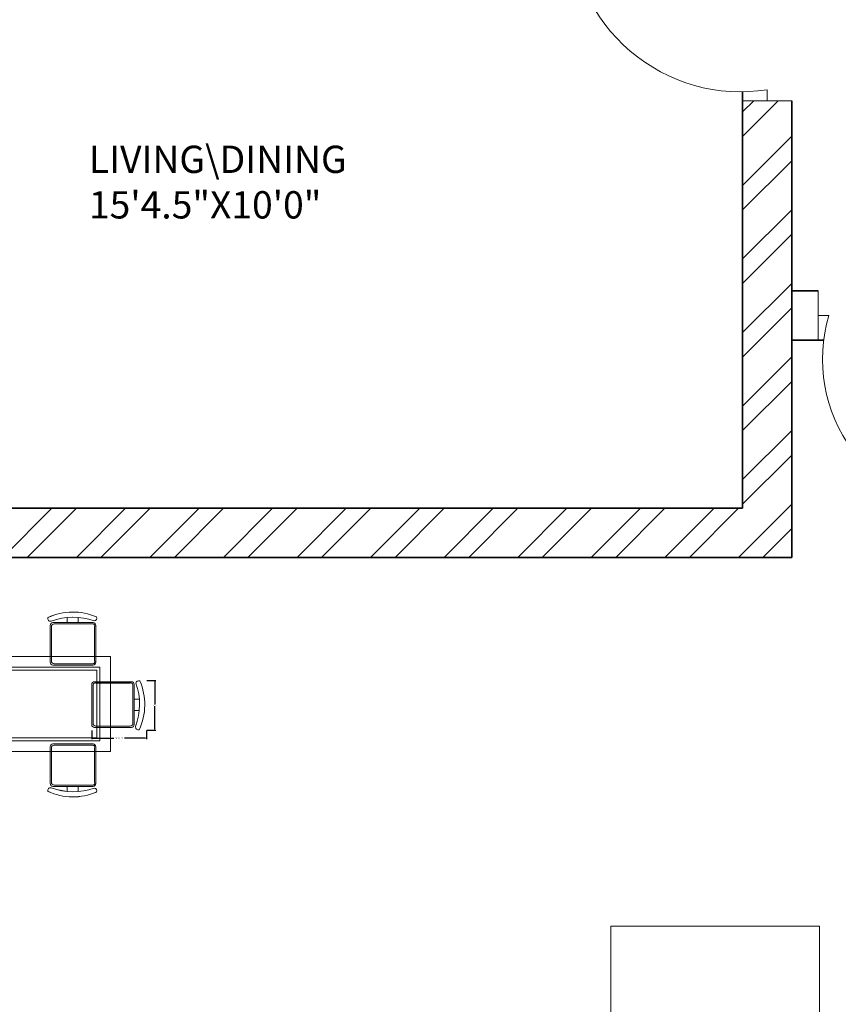
# Model space of a CAD drawing. Units: inches. Extents: x 2120 to 4013, y 1390 to 3019.
# Tile 14 of 59: x 2448 to 2598, y 1784 to 1964. Entities that reach past the tile are written whole.
import ezdxf

# ---------------------------------------------------------------- set-up
doc = ezdxf.new("R2010")
doc.units = ezdxf.units.IN
for name, color, linetype, lineweight in [('A-ANNO-DIMS', 2, 'Continuous', 18), ('A-AREA-IDEN', 7, 'Continuous', 18), ('A-DOOR', 3, 'Continuous', 18), ('A-FURN', 8, 'Continuous', 13), ('A-WALL', 7, 'Continuous', 35), ('A-WALL-PATT', 252, 'Continuous', 13)]:
    doc.layers.add(name, color=color, linetype=linetype, lineweight=lineweight)
doc.styles.get("Standard").update_dxf_attribs({"font": 'arial.ttf'})
doc.dimstyles.get("Standard").update_dxf_attribs({"dimtxt": 0.18, "dimasz": 0.18, "dimexe": 0.18, "dimexo": 0.0625, "dimgap": 0.09, "dimtad": 0, "dimtih": 1, "dimtoh": 1, "dimdec": 4, "dimzin": 0, "dimdsep": 46, "dimtxsty": 'Standard', "dimcen": 0.09, "dimadec": 0, "dimazin": 0, "dimtfac": 1, "dimtdec": 4, "dimtofl": 0, "dimtmove": 0, "dimatfit": 3, "dimfxl": 1, "dimtolj": 1, "dimtzin": 0, "dimarcsym": 0})

# ---------------------------------------------------------------- blocks, each defined once
blk = doc.blocks.new('DOOR-SWING-36IN-98p95DEG')
for p, q in [((31.5, 34.77), (40.5, 34.77)), ((40.5, 34.77), (36, 34.77)), ((36, 34.77), (36, 32.77)), ((36, 32.77), (0, 32.77)), ((36, 0), (36, 2)), ((31.5, 0), (40.5, 0)), ((40.5, 0), (36, 0))]:
    blk.add_line(p, q)
blk.add_arc((31.15, 32.77), 31.15, 180, 278.9496)
blk = doc.blocks.new('DOOR-SWING-36IN-106p79DEG')
for p, q in [((0, 40.5), (0, 31.5)), ((30.74, 31.5), (30.74, 40.5)), ((30.74, 40.5), (30.74, 36)), ((0, 31.5), (0, 36)), ((0, 36), (2, 36)), ((30.74, 36), (28.74, 36)), ((28.74, 36), (28.74, 0))]:
    blk.add_line(p, q)
blk.add_arc((28.74, 27.93), 27.93, 163.2075, 270)
blk = doc.blocks.new('TABLE-DINING')
for points in [[(0, 17.41), (29.01, 17.41), (29.01, 0), (0, 0)], [(1.93, 15.47), (27.08, 15.47), (27.08, 1.93), (1.93, 1.93)], [(2.51, 14.89), (26.5, 14.89), (26.5, 2.51), (2.51, 2.51)]]:
    blk.add_lwpolyline(points, close=True)
blk = doc.blocks.new('TABLE-COFFEE')
blk.add_lwpolyline([(0, 38.19), (21.88, 38.19), (21.88, 0), (0, 0)], close=True)
blk = doc.blocks.new('CHAIR-DINING-01')
for points in [[(1.68, 0.62, -0.578392), (1.02, 0.02, -0.214524), (0.9, 8.94, -0.552014), (1.62, 8.52, 0.175809), (1.68, 0.62)], [(1.93, 8.29, -0.414214), (2.45, 8.81), (9.19, 8.81, -0.414214), (9.7, 8.29), (9.7, 0.96, -0.414214), (9.19, 0.45), (2.45, 0.45, -0.414214), (1.93, 0.96), (1.93, 8.29)], [(1.93, 3.54), (1.01, 3.54, 0.064759)]]:
    blk.add_lwpolyline(points, format="xyb")
blk.add_lwpolyline([(2.16, 8.29), (2.16, 1.19, 0.414214), (2.68, 0.68), (8.96, 0.68, 0.414214), (9.47, 1.19), (9.47, 8.29, 0.512069), (8.96, 8.58), (2.68, 8.58, 0.512069)], format="xyb", close=True)
blk.add_lwpolyline([(0.99, 5.59), (1.93, 5.59)])
blk = doc.blocks.new('CHAIR-DINING-02')
for points in [[(7.77, 8.29, 0.414214), (7.26, 8.81), (0.51, 8.81, 0.414214), (0, 8.29), (0, 0.96, 0.414214), (0.51, 0.45), (7.26, 0.45, 0.414214), (7.77, 0.96), (7.77, 8.29)], [(8.09, 8.52, -0.175809), (8.03, 0.62, 0.578392), (8.69, 0.02, 0.214524), (8.81, 8.94, 0.552014), (8.09, 8.52, -0.065079)], [(7.77, 3.54), (8.7, 3.54, -0.064759)]]:
    blk.add_lwpolyline(points, format="xyb")
blk.add_lwpolyline([(7.54, 8.29), (7.54, 1.19, -0.414214), (7.03, 0.68), (0.74, 0.68, -0.414214), (0.23, 1.19), (0.23, 8.29, -0.512069), (0.74, 8.58), (7.03, 8.58, -0.512069)], format="xyb", close=True)
blk.add_lwpolyline([(8.72, 5.59), (7.77, 5.59)])
blk = doc.blocks.new('CHAIR-DINING-03')
for points in [[(8.29, 1.93, 0.414214), (8.81, 2.45), (8.81, 9.19, 0.414214), (8.29, 9.7), (0.96, 9.7, 0.414214), (0.45, 9.19), (0.45, 2.45, 0.414214), (0.96, 1.93), (8.29, 1.93)], [(3.54, 1.93), (3.54, 1.01, -0.064759)], [(8.52, 1.62, -0.175809), (0.62, 1.68, 0.578392), (0.02, 1.02, 0.214524), (8.94, 0.9, 0.552014), (8.52, 1.62, -0.065079)]]:
    blk.add_lwpolyline(points, format="xyb")
blk.add_lwpolyline([(8.29, 2.16), (1.19, 2.16, -0.414214), (0.68, 2.68), (0.68, 8.96, -0.414214), (1.19, 9.47), (8.29, 9.47, -0.512069), (8.58, 8.96), (8.58, 2.68, -0.512069)], format="xyb", close=True)
blk.add_lwpolyline([(5.59, 0.99), (5.59, 1.93)])
blk = doc.blocks.new('*D83')
at = {"layer": 'A-ANNO-DIMS', "color": 0, "lineweight": -2, "transparency": 16777216}
for p, q in [((2461.05, 1833.87), (2461.05, 1832.25)), ((2471.1, 1833.87), (2471.1, 1832.25)), ((2461.23, 1832.43), (2465.12, 1832.43)), ((2470.92, 1832.43), (2467.03, 1832.43))]:
    blk.add_line(p, q, dxfattribs=at)
at = {"layer": 'A-ANNO-DIMS', "color": 0, "transparency": 16777216}
for points in [[(2461.23, 1832.46), (2461.23, 1832.4), (2461.05, 1832.43)], [(2470.92, 1832.46), (2470.92, 1832.4), (2471.1, 1832.43)]]:
    blk.add_solid(points, dxfattribs=at)
at = {"layer": 'Defpoints', "color": 0, "transparency": 16777216}
for p in [(2461.05, 1833.93), (2471.1, 1833.93), (2471.1, 1832.43)]:
    blk.add_point(p, dxfattribs=at)
at = {"layer": 'A-ANNO-DIMS', "color": 0, "transparency": 16777216, "insert": (2466.08, 1832.43), "char_height": 0.18, "attachment_point": 5}
blk.add_mtext('\\A1;CHAIR 10 TYP.', dxfattribs=at)
blk = doc.blocks.new('*D84')
at = {"layer": 'A-ANNO-DIMS', "color": 0, "lineweight": -2, "transparency": 16777216}
for p, q in [((2471.16, 1842.99), (2472.78, 1842.99)), ((2472.6, 1842.81), (2472.6, 1838.64)), ((2472.6, 1834.11), (2472.6, 1838.28)), ((2471.16, 1833.93), (2472.78, 1833.93))]:
    blk.add_line(p, q, dxfattribs=at)
at = {"layer": 'A-ANNO-DIMS', "color": 0, "transparency": 16777216}
for points in [[(2472.57, 1842.81), (2472.63, 1842.81), (2472.6, 1842.99)], [(2472.57, 1834.11), (2472.63, 1834.11), (2472.6, 1833.93)]]:
    blk.add_solid(points, dxfattribs=at)
at = {"layer": 'Defpoints', "color": 0, "transparency": 16777216}
for p in [(2471.1, 1842.99), (2472.6, 1842.99), (2471.1, 1833.93)]:
    blk.add_point(p, dxfattribs=at)
at = {"layer": 'A-ANNO-DIMS', "color": 0, "transparency": 16777216, "insert": (2472.6, 1838.46), "char_height": 0.18, "attachment_point": 5}
blk.add_mtext('\\A1;9 TYP.', dxfattribs=at)

msp = doc.modelspace()

# ---------------------------------------------------------------- hatches: boundary and pattern name
at = {"layer": 'A-WALL-PATT'}
h = msp.add_hatch(dxfattribs=at)
h.set_pattern_fill('ANSI32', color=256)
h.paths.add_polyline_path([(2271.7331, 2343.531), (2283.3788, 2343.531), (2283.3788, 2348.031), (2283.3788, 2352.5306), (2262.7331, 2352.5306), (2262.7331, 2182.638), (2267.2331, 2182.638), (2271.7331, 2182.638), (2271.7331, 2219.031), (2391.7331, 2219.031), (2391.7331, 2214.189), (2393.9831, 2214.189), (2396.2331, 2214.189), (2396.2331, 2219.031), (2420.2331, 2219.031), (2420.2331, 2225.7535), (2417.2197, 2225.7535), (2415.7331, 2225.7535), (2415.7331, 2223.5306), (2271.7331, 2223.5306)])
h.paths.add_polyline_path([(2380.0942, 2352.5306), (2343.3788, 2352.5306), (2343.3788, 2343.531), (2363.2331, 2343.531), (2363.2331, 2288.8489), (2365.4831, 2288.8489), (2367.7331, 2288.8489), (2367.7331, 2343.531), (2380.0942, 2343.531)], flags=17)
h.paths.add_polyline_path([(2432.4339, 2352.5306), (2404.0943, 2352.5306), (2404.0943, 2343.531), (2415.7331, 2343.531), (2415.7331, 2264.0306), (2367.7331, 2264.0306), (2367.7331, 2266.4872), (2363.2331, 2266.4872), (2363.2331, 2259.531), (2367.7331, 2259.531), (2415.7331, 2259.531), (2415.7331, 2255.0658), (2420.2331, 2255.0658), (2420.2331, 2259.531), (2424.5717, 2259.531), (2424.5717, 2261.781), (2424.5717, 2264.0306), (2420.2331, 2264.0306), (2420.2331, 2343.531), (2432.4339, 2343.531)])
h.paths.add_polyline_path([(2508.9115, 2352.5306), (2456.4339, 2352.5306), (2456.4339, 2343.531), (2468.2331, 2343.531), (2468.2331, 2264.0306), (2448.0487, 2264.0306), (2448.0487, 2259.531), (2468.2331, 2259.531), (2468.2331, 2255.5496), (2472.7331, 2255.5496), (2472.7331, 2343.531), (2508.9115, 2343.531)])
h.paths.add_polyline_path([(2637.7331, 2352.5306), (2544.9116, 2352.5306), (2544.9116, 2343.531), (2589.7331, 2343.531), (2633.2331, 2343.531), (2637.7331, 2343.531)])
h.paths.add_polyline_path([(2594.2331, 2343.5306), (2589.7331, 2343.5306), (2589.7331, 2259.5306), (2589.7331, 2252.4915), (2591.9831, 2252.4915), (2594.2331, 2252.4915)])
h.paths.add_polyline_path([(2637.7331, 2223.5306), (2594.2331, 2223.5306), (2594.2331, 2230.1988), (2591.9831, 2230.1988), (2589.7331, 2230.1988), (2589.7331, 2223.5306), (2472.7331, 2223.5306), (2468.2331, 2223.5306), (2468.2331, 2219.031), (2628.7331, 2219.031), (2628.7331, 2138.031), (2637.7331, 2138.031)])
h.paths.add_polyline_path([(3822.6535, 2458.4402), (3874.9468, 2458.4402), (3874.9468, 2476.9866), (3822.6535, 2476.9866)], flags=9)
h.paths.add_polyline_path([(3834.6921, 2781.8174), (3935.9206, 2781.8174), (3935.9206, 2800.3638), (3834.6921, 2800.3638)], flags=9)
h.paths.add_polyline_path([(3832.2843, 2837.9683), (3884.5776, 2837.9683), (3884.5776, 2856.5146), (3832.2843, 2856.5146)], flags=9)
h.paths.add_polyline_path([(3830.9388, 2861.4782), (3956.8958, 2861.4782), (3956.8958, 2880.0245), (3830.9388, 2880.0245)], flags=9)
h.paths.add_polyline_path([(3870.6966, 2352.5752), (3887.9272, 2352.5752), (3887.9272, 2377.3037), (3870.6966, 2377.3037)], flags=9)
h.paths.add_polyline_path([(3289.2701, 2413.161), (3435.2223, 2413.161), (3435.2223, 2450.2538), (3289.2701, 2450.2538)], flags=9)
h.paths.add_polyline_path([(2487.6944, 2414.3601), (2637.8335, 2414.3601), (2637.8335, 2451.4528), (2487.6944, 2451.4528)], flags=9)
h.paths.add_polyline_path([(2567.3724, 1457.9199), (2815.296, 1457.9199), (2815.296, 1495.0127), (2567.3724, 1495.0127)], flags=9)
h.paths.add_polyline_path([(2655.3825, 2093.2363), (2685.9555, 2093.2363), (2685.9555, 2111.8937), (2655.3825, 2111.8937)], flags=9)
h.paths.add_polyline_path([(2543.9218, 1550.6671), (2587.8406, 1550.6671), (2587.8406, 1569.3244), (2543.9218, 1569.3244)], flags=9)
h.paths.add_polyline_path([(2905.1384, 1543.8113), (2949.0572, 1543.8113), (2949.0572, 1562.4686), (2905.1384, 1562.4686)], flags=9)
h.paths.add_polyline_path([(2736.4118, 1702.4736), (2784.2153, 1702.4736), (2784.2153, 1721.1309), (2736.4118, 1721.1309)], flags=9)
h.paths.add_polyline_path([(2912.8666, 1710.4168), (2951.707, 1710.4168), (2951.707, 1729.0741), (2912.8666, 1729.0741)], flags=9)
h.paths.add_polyline_path([(2923.5785, 1763.5038), (2959.7279, 1763.5038), (2959.7279, 1782.1611), (2923.5785, 1782.1611)], flags=9)
h.paths.add_polyline_path([(2925.2114, 1809.6137), (2967.1861, 1809.6137), (2967.1861, 1828.271), (2925.2114, 1828.271)], flags=9)
h.paths.add_polyline_path([(2996.2711, 1878.9003), (2996.2711, 1913.109), (2977.6138, 1913.109), (2977.6138, 1878.9003)], flags=9)
h.paths.add_polyline_path([(2883.0859, 1895.7192), (2927.1855, 1895.7192), (2927.1855, 1914.3766), (2883.0859, 1914.3766)], flags=9)
h.paths.add_polyline_path([(2787.3924, 1810.8013), (2841.0213, 1810.8013), (2841.0213, 1829.4587), (2787.3924, 1829.4587)], flags=9)
h.paths.add_polyline_path([(2775.6399, 2101.7395), (2829.2689, 2101.7395), (2829.2689, 2120.3968), (2775.6399, 2120.3968)], flags=9)
h.paths.add_polyline_path([(2913.0263, 2075.817), (2951.8667, 2075.817), (2951.8667, 2094.4744), (2913.0263, 2094.4744)], flags=9)
h.paths.add_polyline_path([(2929.966, 2133.3669), (2966.1154, 2133.3669), (2966.1154, 2152.0243), (2929.966, 2152.0243)], flags=9)
h.paths.add_polyline_path([(2932.7502, 2182.6088), (2968.8996, 2182.6088), (2968.8996, 2201.2662), (2932.7502, 2201.2662)], flags=9)
h.paths.add_polyline_path([(2996.0681, 2266.3173), (2996.0681, 2300.5261), (2977.4108, 2300.5261), (2977.4108, 2266.3173)], flags=9)
h.paths.add_polyline_path([(2885.1039, 2279.2186), (2929.2035, 2279.2186), (2929.2035, 2297.8759), (2885.1039, 2297.8759)], flags=9)
h.paths.add_polyline_path([(2735.7042, 2218.3197), (2783.5078, 2218.3197), (2783.5078, 2236.9771), (2735.7042, 2236.9771)], flags=9)
h.paths.add_polyline_path([(2635.6049, 2044.0085), (2648.9678, 2044.0085), (2648.9678, 2054.312), (2635.6049, 2054.312)], flags=9)
h.paths.add_polyline_path([(2714.0148, 1923.0473), (2727.3777, 1923.0473), (2727.3777, 1933.3508), (2714.0148, 1933.3508)], flags=9)
h.paths.add_polyline_path([(2709.0345, 1988.1628), (2722.3974, 1988.1628), (2722.3974, 1998.4663), (2709.0345, 1998.4663)], flags=9)
h.paths.add_polyline_path([(2592.8935, 1962.1763), (2606.2564, 1962.1763), (2606.2564, 1972.4799), (2592.8935, 1972.4799)], flags=9)
h.paths.add_polyline_path([(2618.3996, 1985.9724), (2644.1942, 1985.9724), (2644.1942, 1996.2759), (2618.3996, 1996.2759)], flags=9)
h.paths.add_polyline_path([(2601.279, 1920.5869), (2614.6419, 1920.5869), (2614.6419, 1930.8904), (2601.279, 1930.8904)], flags=9)
h.paths.add_polyline_path([(2692.3278, 1932.7645), (2704.5311, 1932.7645), (2704.5311, 1943.0681), (2692.3278, 1943.0681)], flags=9)
h.paths.add_polyline_path([(2311.122, 1672.7318), (2355.0408, 1672.7318), (2355.0408, 1691.3892), (2311.122, 1691.3892)], flags=9)
h.paths.add_polyline_path([(2456.2551, 1632.3198), (2492.4796, 1632.3198), (2492.4796, 1650.9772), (2456.2551, 1650.9772)], flags=9)
h.paths.add_polyline_path([(2401.0766, 1631.4793), (2437.301, 1631.4793), (2437.301, 1650.1367), (2401.0766, 1650.1367)], flags=9)
h.paths.add_polyline_path([(2546.7054, 1700.9235), (2594.509, 1700.9235), (2594.509, 1719.5809), (2546.7054, 1719.5809)], flags=9)
h.paths.add_polyline_path([(2445.4866, 1766.9937), (2497.5261, 1766.9937), (2497.5261, 1785.651), (2445.4866, 1785.651)], flags=9)
h.paths.add_polyline_path([(2287.9992, 1739.7675), (2326.8396, 1739.7675), (2326.8396, 1758.4248), (2287.9992, 1758.4248)], flags=9)
h.paths.add_polyline_path([(2458.5279, 1924.7607), (2510.5675, 1924.7607), (2510.5675, 1943.4181), (2458.5279, 1943.4181)], flags=9)
h.paths.add_polyline_path([(2309.2811, 1902.7642), (2345.4305, 1902.7642), (2345.4305, 1921.4215), (2309.2811, 1921.4215)], flags=9)
h.paths.add_polyline_path([(2490.7554, 2018.9392), (2530.7896, 2018.9392), (2530.7896, 2037.5965), (2490.7554, 2037.5965)], flags=9)
h.paths.add_polyline_path([(2402.143, 2024.7393), (2438.5414, 2024.7393), (2438.5414, 2043.3966), (2402.143, 2043.3966)], flags=9)
h.paths.add_polyline_path([(2287.856, 1931.7926), (2326.6964, 1931.7926), (2326.6964, 1950.4499), (2287.856, 1950.4499)], flags=9)
h.paths.add_polyline_path([(2281.7979, 2193.5771), (2320.6383, 2193.5771), (2320.6383, 2212.2344), (2281.7979, 2212.2344)], flags=25)
h.paths.add_polyline_path([(2484.0754, 2093.892), (2536.115, 2093.892), (2536.115, 2112.5494), (2484.0754, 2112.5494)], flags=9)
h.paths.add_polyline_path([(2624.7948, 2281.8639), (2624.7948, 2311.4137), (2606.1375, 2311.4137), (2606.1375, 2281.8639)], flags=9)
h.paths.add_polyline_path([(2507.5036, 2290.3639), (2541.934, 2290.3639), (2541.934, 2309.0212), (2507.5036, 2309.0212)], flags=9)
h.paths.add_polyline_path([(2423.1076, 2285.2202), (2459.332, 2285.2202), (2459.332, 2303.8776), (2423.1076, 2303.8776)], flags=9)
h.paths.add_polyline_path([(2374.5467, 2289.6272), (2410.7711, 2289.6272), (2410.7711, 2308.2846), (2374.5467, 2308.2846)], flags=25)
h.paths.add_polyline_path([(2277.4907, 2227.5651), (2316.3311, 2227.5651), (2316.3311, 2246.2224), (2277.4907, 2246.2224)], flags=25)
h.paths.add_polyline_path([(2655.3825, 2093.2367), (2685.9555, 2093.2367), (2685.9555, 2111.894), (2655.3825, 2111.894)], flags=9)
h.paths.add_polyline_path([(2543.9217, 1550.6674), (2587.8406, 1550.6674), (2587.8406, 1569.3247), (2543.9217, 1569.3247)], flags=9)
h.paths.add_polyline_path([(2905.1384, 1543.8116), (2949.0572, 1543.8116), (2949.0572, 1562.4689), (2905.1384, 1562.4689)], flags=9)
h.paths.add_polyline_path([(2736.4118, 1702.4739), (2784.2153, 1702.4739), (2784.2153, 1721.1312), (2736.4118, 1721.1312)], flags=9)
h.paths.add_polyline_path([(2912.8666, 1710.4171), (2951.707, 1710.4171), (2951.707, 1729.0744), (2912.8666, 1729.0744)], flags=9)
h.paths.add_polyline_path([(2923.5785, 1763.5041), (2959.7279, 1763.5041), (2959.7279, 1782.1614), (2923.5785, 1782.1614)], flags=9)
h.paths.add_polyline_path([(2925.2114, 1809.614), (2967.1861, 1809.614), (2967.1861, 1828.2713), (2925.2114, 1828.2713)], flags=9)
h.paths.add_polyline_path([(2996.2711, 1878.9006), (2996.2711, 1913.1094), (2977.6137, 1913.1094), (2977.6137, 1878.9006)], flags=9)
h.paths.add_polyline_path([(2883.0859, 1895.7195), (2927.1855, 1895.7195), (2927.1855, 1914.3769), (2883.0859, 1914.3769)], flags=9)
h.paths.add_polyline_path([(2787.3924, 1810.8016), (2841.0213, 1810.8016), (2841.0213, 1829.459), (2787.3924, 1829.459)], flags=9)
h.paths.add_polyline_path([(2775.6399, 2101.7398), (2829.2688, 2101.7398), (2829.2688, 2120.3971), (2775.6399, 2120.3971)], flags=9)
h.paths.add_polyline_path([(2913.0263, 2075.8173), (2951.8667, 2075.8173), (2951.8667, 2094.4747), (2913.0263, 2094.4747)], flags=9)
h.paths.add_polyline_path([(2929.966, 2133.3672), (2966.1154, 2133.3672), (2966.1154, 2152.0246), (2929.966, 2152.0246)], flags=9)
h.paths.add_polyline_path([(2932.7502, 2182.6091), (2968.8996, 2182.6091), (2968.8996, 2201.2665), (2932.7502, 2201.2665)], flags=9)
h.paths.add_polyline_path([(2996.0681, 2266.3176), (2996.0681, 2300.5264), (2977.4108, 2300.5264), (2977.4108, 2266.3176)], flags=9)
h.paths.add_polyline_path([(2885.1039, 2279.2189), (2929.2035, 2279.2189), (2929.2035, 2297.8762), (2885.1039, 2297.8762)], flags=9)
h.paths.add_polyline_path([(2735.7042, 2218.32), (2783.5078, 2218.32), (2783.5078, 2236.9774), (2735.7042, 2236.9774)], flags=9)
h.paths.add_polyline_path([(2635.6048, 2044.0088), (2648.9677, 2044.0088), (2648.9677, 2054.3123), (2635.6048, 2054.3123)], flags=9)
h.paths.add_polyline_path([(2714.0148, 1923.0476), (2727.3777, 1923.0476), (2727.3777, 1933.3511), (2714.0148, 1933.3511)], flags=9)
h.paths.add_polyline_path([(2709.0345, 1988.1631), (2722.3974, 1988.1631), (2722.3974, 1998.4666), (2709.0345, 1998.4666)], flags=9)
h.paths.add_polyline_path([(2592.8935, 1962.1766), (2606.2564, 1962.1766), (2606.2564, 1972.4802), (2592.8935, 1972.4802)], flags=9)
h.paths.add_polyline_path([(2618.3995, 1985.9727), (2644.1942, 1985.9727), (2644.1942, 1996.2762), (2618.3995, 1996.2762)], flags=9)
h.paths.add_polyline_path([(2601.279, 1920.5872), (2614.6419, 1920.5872), (2614.6419, 1930.8908), (2601.279, 1930.8908)], flags=9)
h.paths.add_polyline_path([(2692.3278, 1932.7648), (2704.5311, 1932.7648), (2704.5311, 1943.0684), (2692.3278, 1943.0684)], flags=9)
h.paths.add_polyline_path([(2311.122, 1672.7321), (2355.0408, 1672.7321), (2355.0408, 1691.3895), (2311.122, 1691.3895)], flags=9)
h.paths.add_polyline_path([(2456.2551, 1632.3201), (2492.4795, 1632.3201), (2492.4795, 1650.9775), (2456.2551, 1650.9775)], flags=9)
h.paths.add_polyline_path([(2401.0766, 1631.4796), (2437.301, 1631.4796), (2437.301, 1650.137), (2401.0766, 1650.137)], flags=9)
h.paths.add_polyline_path([(2546.7054, 1700.9238), (2594.509, 1700.9238), (2594.509, 1719.5812), (2546.7054, 1719.5812)], flags=9)
h.paths.add_polyline_path([(2445.4866, 1766.994), (2497.5261, 1766.994), (2497.5261, 1785.6513), (2445.4866, 1785.6513)], flags=9)
h.paths.add_polyline_path([(2287.9992, 1739.7678), (2326.8396, 1739.7678), (2326.8396, 1758.4251), (2287.9992, 1758.4251)], flags=9)
h.paths.add_polyline_path([(2458.5279, 1924.7611), (2510.5675, 1924.7611), (2510.5675, 1943.4184), (2458.5279, 1943.4184)], flags=9)
h.paths.add_polyline_path([(2309.2811, 1902.7645), (2345.4305, 1902.7645), (2345.4305, 1921.4218), (2309.2811, 1921.4218)], flags=9)
h.paths.add_polyline_path([(2490.7554, 2018.9395), (2530.7895, 2018.9395), (2530.7895, 2037.5968), (2490.7554, 2037.5968)], flags=9)
h.paths.add_polyline_path([(2402.143, 2024.7396), (2438.5413, 2024.7396), (2438.5413, 2043.3969), (2402.143, 2043.3969)], flags=9)
h.paths.add_polyline_path([(2287.856, 1931.7929), (2326.6964, 1931.7929), (2326.6964, 1950.4502), (2287.856, 1950.4502)], flags=9)
h.paths.add_polyline_path([(2281.7979, 2193.5774), (2320.6383, 2193.5774), (2320.6383, 2212.2347), (2281.7979, 2212.2347)], flags=25)
h.paths.add_polyline_path([(2484.0754, 2093.8924), (2536.115, 2093.8924), (2536.115, 2112.5497), (2484.0754, 2112.5497)], flags=9)
h.paths.add_polyline_path([(2624.7948, 2281.8642), (2624.7948, 2311.414), (2606.1374, 2311.414), (2606.1374, 2281.8642)], flags=9)
h.paths.add_polyline_path([(2507.5035, 2290.3642), (2541.934, 2290.3642), (2541.934, 2309.0215), (2507.5035, 2309.0215)], flags=9)
h.paths.add_polyline_path([(2423.1075, 2285.2205), (2459.332, 2285.2205), (2459.332, 2303.8779), (2423.1075, 2303.8779)], flags=9)
h.paths.add_polyline_path([(2374.5467, 2289.6275), (2410.7711, 2289.6275), (2410.7711, 2308.2849), (2374.5467, 2308.2849)], flags=25)
h.paths.add_polyline_path([(2277.4907, 2227.5654), (2316.3311, 2227.5654), (2316.3311, 2246.2227), (2277.4907, 2246.2227)], flags=25)
h = msp.add_hatch(dxfattribs=at)
h.set_pattern_fill('ANSI32', color=256)
h.paths.add_polyline_path([(2271.7331, 1980.389), (2262.7331, 1980.389), (2262.7331, 1912.8434), (2267.2331, 1912.8434), (2271.7331, 1912.8434), (2271.7331, 1922.531), (2351.2331, 1922.531), (2351.2331, 1901.4728), (2355.7331, 1901.4728), (2355.7331, 1922.531), (2357.9815, 1922.531), (2357.9815, 1926.5306), (2271.7331, 1926.5306)])
h.paths.add_polyline_path([(2589.2331, 1949.1622), (2584.7331, 1949.1622), (2580.2331, 1949.1622), (2580.2331, 1874.5306), (2355.7331, 1874.5306), (2355.7331, 1880.1922), (2351.2331, 1880.1922), (2351.2331, 1874.5306), (2271.7331, 1874.5306), (2271.7331, 1888.8431), (2262.7331, 1888.8431), (2262.7331, 1842.2909), (2267.2331, 1842.2909), (2271.7331, 1842.2909), (2271.7331, 1865.531), (2415.7331, 1865.531), (2415.7331, 1779.7286), (2420.2331, 1779.7286), (2420.2331, 1865.531), (2589.2331, 1865.531)])
h.paths.add_polyline_path([(2271.7331, 1782.2906), (2262.7331, 1782.2906), (2262.7331, 1711.4639), (2267.2331, 1711.4639), (2271.7331, 1711.4639), (2271.7331, 1738.031), (2420.2331, 1738.031), (2420.2331, 1742.531), (2420.2331, 1747.3376), (2417.9831, 1747.3376), (2415.7331, 1747.3376), (2415.7331, 1742.5306), (2271.7331, 1742.5306)])
h.paths.add_polyline_path([(2271.7331, 1627.031), (2362.3957, 1627.031), (2362.3957, 1629.281), (2362.3957, 1631.5306), (2271.7331, 1631.5306), (2271.7331, 1675.4636), (2262.7331, 1675.4636), (2262.7331, 1581.531), (2405.3032, 1581.531), (2405.3032, 1586.031), (2405.3032, 1590.5306), (2396.2331, 1590.5306), (2396.2331, 1691.4513), (2418.7206, 1691.4513), (2418.7206, 1695.951), (2396.2331, 1695.951), (2391.7331, 1695.951), (2391.7331, 1631.5306), (2386.7425, 1631.5306), (2386.7425, 1629.2806), (2386.7425, 1627.031), (2391.7331, 1627.031), (2391.7331, 1586.1709), (2271.7331, 1586.1709)])
h.paths.add_polyline_path([(2459.6703, 1590.5306), (2429.3032, 1590.5306), (2429.3032, 1581.531), (2459.6703, 1581.531), (2459.6703, 1586.031)])
h.paths.add_polyline_path([(2501.2331, 1590.531), (2501.2331, 1665.0195), (2498.9831, 1665.0195), (2496.7331, 1665.0195), (2496.7331, 1590.5306), (2483.8201, 1590.5306), (2483.8201, 1590.1579), (2483.6704, 1590.1579), (2483.6704, 1581.531), (2505.0196, 1581.531), (2505.0196, 1583.781), (2505.0196, 1586.0306), (2501.2331, 1586.0306)])
h.paths.add_polyline_path([(2544.1361, 1583.781), (2544.1361, 1586.0306), (2527.1368, 1586.0306), (2527.1368, 1583.7806), (2527.1368, 1581.531), (2544.1361, 1581.531)])
h.paths.add_polyline_path([(3822.6535, 2458.4402), (3874.9468, 2458.4402), (3874.9468, 2476.9866), (3822.6535, 2476.9866)], flags=9)
h.paths.add_polyline_path([(3834.6921, 2781.8174), (3935.9206, 2781.8174), (3935.9206, 2800.3638), (3834.6921, 2800.3638)], flags=9)
h.paths.add_polyline_path([(3832.2843, 2837.9683), (3884.5776, 2837.9683), (3884.5776, 2856.5146), (3832.2843, 2856.5146)], flags=9)
h.paths.add_polyline_path([(3830.9388, 2861.4782), (3956.8958, 2861.4782), (3956.8958, 2880.0245), (3830.9388, 2880.0245)], flags=9)
h.paths.add_polyline_path([(3870.6966, 2352.5752), (3887.9272, 2352.5752), (3887.9272, 2377.3037), (3870.6966, 2377.3037)], flags=9)
h.paths.add_polyline_path([(3289.2701, 2413.161), (3435.2223, 2413.161), (3435.2223, 2450.2538), (3289.2701, 2450.2538)], flags=9)
h.paths.add_polyline_path([(2487.6944, 2414.3601), (2637.8335, 2414.3601), (2637.8335, 2451.4528), (2487.6944, 2451.4528)], flags=9)
h.paths.add_polyline_path([(2567.3724, 1457.9199), (2815.296, 1457.9199), (2815.296, 1495.0127), (2567.3724, 1495.0127)], flags=9)
h.paths.add_polyline_path([(2655.3825, 2093.2363), (2685.9555, 2093.2363), (2685.9555, 2111.8937), (2655.3825, 2111.8937)], flags=9)
h.paths.add_polyline_path([(2543.9218, 1550.6671), (2587.8406, 1550.6671), (2587.8406, 1569.3244), (2543.9218, 1569.3244)], flags=9)
h.paths.add_polyline_path([(2905.1384, 1543.8113), (2949.0572, 1543.8113), (2949.0572, 1562.4686), (2905.1384, 1562.4686)], flags=9)
h.paths.add_polyline_path([(2736.4118, 1702.4736), (2784.2153, 1702.4736), (2784.2153, 1721.1309), (2736.4118, 1721.1309)], flags=9)
h.paths.add_polyline_path([(2912.8666, 1710.4168), (2951.707, 1710.4168), (2951.707, 1729.0741), (2912.8666, 1729.0741)], flags=9)
h.paths.add_polyline_path([(2923.5785, 1763.5038), (2959.7279, 1763.5038), (2959.7279, 1782.1611), (2923.5785, 1782.1611)], flags=9)
h.paths.add_polyline_path([(2925.2114, 1809.6137), (2967.1861, 1809.6137), (2967.1861, 1828.271), (2925.2114, 1828.271)], flags=9)
h.paths.add_polyline_path([(2996.2711, 1878.9003), (2996.2711, 1913.109), (2977.6138, 1913.109), (2977.6138, 1878.9003)], flags=9)
h.paths.add_polyline_path([(2883.0859, 1895.7192), (2927.1855, 1895.7192), (2927.1855, 1914.3766), (2883.0859, 1914.3766)], flags=9)
h.paths.add_polyline_path([(2787.3924, 1810.8013), (2841.0213, 1810.8013), (2841.0213, 1829.4587), (2787.3924, 1829.4587)], flags=9)
h.paths.add_polyline_path([(2775.6399, 2101.7395), (2829.2689, 2101.7395), (2829.2689, 2120.3968), (2775.6399, 2120.3968)], flags=9)
h.paths.add_polyline_path([(2913.0263, 2075.817), (2951.8667, 2075.817), (2951.8667, 2094.4744), (2913.0263, 2094.4744)], flags=9)
h.paths.add_polyline_path([(2929.966, 2133.3669), (2966.1154, 2133.3669), (2966.1154, 2152.0243), (2929.966, 2152.0243)], flags=9)
h.paths.add_polyline_path([(2932.7502, 2182.6088), (2968.8996, 2182.6088), (2968.8996, 2201.2662), (2932.7502, 2201.2662)], flags=9)
h.paths.add_polyline_path([(2996.0681, 2266.3173), (2996.0681, 2300.5261), (2977.4108, 2300.5261), (2977.4108, 2266.3173)], flags=9)
h.paths.add_polyline_path([(2885.1039, 2279.2186), (2929.2035, 2279.2186), (2929.2035, 2297.8759), (2885.1039, 2297.8759)], flags=9)
h.paths.add_polyline_path([(2735.7042, 2218.3197), (2783.5078, 2218.3197), (2783.5078, 2236.9771), (2735.7042, 2236.9771)], flags=9)
h.paths.add_polyline_path([(2635.6049, 2044.0085), (2648.9678, 2044.0085), (2648.9678, 2054.312), (2635.6049, 2054.312)], flags=9)
h.paths.add_polyline_path([(2714.0148, 1923.0473), (2727.3777, 1923.0473), (2727.3777, 1933.3508), (2714.0148, 1933.3508)], flags=9)
h.paths.add_polyline_path([(2709.0345, 1988.1628), (2722.3974, 1988.1628), (2722.3974, 1998.4663), (2709.0345, 1998.4663)], flags=9)
h.paths.add_polyline_path([(2592.8935, 1962.1763), (2606.2564, 1962.1763), (2606.2564, 1972.4799), (2592.8935, 1972.4799)], flags=9)
h.paths.add_polyline_path([(2618.3996, 1985.9724), (2644.1942, 1985.9724), (2644.1942, 1996.2759), (2618.3996, 1996.2759)], flags=9)
h.paths.add_polyline_path([(2601.279, 1920.5869), (2614.6419, 1920.5869), (2614.6419, 1930.8904), (2601.279, 1930.8904)], flags=9)
h.paths.add_polyline_path([(2692.3278, 1932.7645), (2704.5311, 1932.7645), (2704.5311, 1943.0681), (2692.3278, 1943.0681)], flags=9)
h.paths.add_polyline_path([(2311.122, 1672.7318), (2355.0408, 1672.7318), (2355.0408, 1691.3892), (2311.122, 1691.3892)], flags=25)
h.paths.add_polyline_path([(2456.2551, 1632.3198), (2492.4796, 1632.3198), (2492.4796, 1650.9772), (2456.2551, 1650.9772)], flags=9)
h.paths.add_polyline_path([(2401.0766, 1631.4793), (2437.301, 1631.4793), (2437.301, 1650.1367), (2401.0766, 1650.1367)], flags=9)
h.paths.add_polyline_path([(2546.7054, 1700.9235), (2594.509, 1700.9235), (2594.509, 1719.5809), (2546.7054, 1719.5809)], flags=9)
h.paths.add_polyline_path([(2445.4866, 1766.9937), (2497.5261, 1766.9937), (2497.5261, 1785.651), (2445.4866, 1785.651)], flags=9)
h.paths.add_polyline_path([(2287.9992, 1739.7675), (2326.8396, 1739.7675), (2326.8396, 1758.4248), (2287.9992, 1758.4248)], flags=24)
h.paths.add_polyline_path([(2458.5279, 1924.7607), (2510.5675, 1924.7607), (2510.5675, 1943.4181), (2458.5279, 1943.4181)], flags=25)
h.paths.add_polyline_path([(2309.2811, 1902.7642), (2345.4305, 1902.7642), (2345.4305, 1921.4215), (2309.2811, 1921.4215)], flags=25)
h.paths.add_polyline_path([(2490.7554, 2018.9392), (2530.7896, 2018.9392), (2530.7896, 2037.5965), (2490.7554, 2037.5965)], flags=9)
h.paths.add_polyline_path([(2402.143, 2024.7393), (2438.5414, 2024.7393), (2438.5414, 2043.3966), (2402.143, 2043.3966)], flags=9)
h.paths.add_polyline_path([(2287.856, 1931.7926), (2326.6964, 1931.7926), (2326.6964, 1950.4499), (2287.856, 1950.4499)], flags=25)
h.paths.add_polyline_path([(2281.7979, 2193.5771), (2320.6383, 2193.5771), (2320.6383, 2212.2344), (2281.7979, 2212.2344)], flags=9)
h.paths.add_polyline_path([(2484.0754, 2093.892), (2536.115, 2093.892), (2536.115, 2112.5494), (2484.0754, 2112.5494)], flags=9)
h.paths.add_polyline_path([(2624.7948, 2281.8639), (2624.7948, 2311.4137), (2606.1375, 2311.4137), (2606.1375, 2281.8639)], flags=9)
h.paths.add_polyline_path([(2507.5036, 2290.3639), (2541.934, 2290.3639), (2541.934, 2309.0212), (2507.5036, 2309.0212)], flags=9)
h.paths.add_polyline_path([(2423.1076, 2285.2202), (2459.332, 2285.2202), (2459.332, 2303.8776), (2423.1076, 2303.8776)], flags=9)
h.paths.add_polyline_path([(2374.5467, 2289.6272), (2410.7711, 2289.6272), (2410.7711, 2308.2846), (2374.5467, 2308.2846)], flags=9)
h.paths.add_polyline_path([(2277.4907, 2227.5651), (2316.3311, 2227.5651), (2316.3311, 2246.2224), (2277.4907, 2246.2224)], flags=9)
h.paths.add_polyline_path([(2655.3825, 2093.2367), (2685.9555, 2093.2367), (2685.9555, 2111.894), (2655.3825, 2111.894)], flags=9)
h.paths.add_polyline_path([(2543.9217, 1550.6674), (2587.8406, 1550.6674), (2587.8406, 1569.3247), (2543.9217, 1569.3247)], flags=9)
h.paths.add_polyline_path([(2905.1384, 1543.8116), (2949.0572, 1543.8116), (2949.0572, 1562.4689), (2905.1384, 1562.4689)], flags=9)
h.paths.add_polyline_path([(2736.4118, 1702.4739), (2784.2153, 1702.4739), (2784.2153, 1721.1312), (2736.4118, 1721.1312)], flags=9)
h.paths.add_polyline_path([(2912.8666, 1710.4171), (2951.707, 1710.4171), (2951.707, 1729.0744), (2912.8666, 1729.0744)], flags=9)
h.paths.add_polyline_path([(2923.5785, 1763.5041), (2959.7279, 1763.5041), (2959.7279, 1782.1614), (2923.5785, 1782.1614)], flags=9)
h.paths.add_polyline_path([(2925.2114, 1809.614), (2967.1861, 1809.614), (2967.1861, 1828.2713), (2925.2114, 1828.2713)], flags=9)
h.paths.add_polyline_path([(2996.2711, 1878.9006), (2996.2711, 1913.1094), (2977.6137, 1913.1094), (2977.6137, 1878.9006)], flags=9)
h.paths.add_polyline_path([(2883.0859, 1895.7195), (2927.1855, 1895.7195), (2927.1855, 1914.3769), (2883.0859, 1914.3769)], flags=9)
h.paths.add_polyline_path([(2787.3924, 1810.8016), (2841.0213, 1810.8016), (2841.0213, 1829.459), (2787.3924, 1829.459)], flags=9)
h.paths.add_polyline_path([(2775.6399, 2101.7398), (2829.2688, 2101.7398), (2829.2688, 2120.3971), (2775.6399, 2120.3971)], flags=9)
h.paths.add_polyline_path([(2913.0263, 2075.8173), (2951.8667, 2075.8173), (2951.8667, 2094.4747), (2913.0263, 2094.4747)], flags=9)
h.paths.add_polyline_path([(2929.966, 2133.3672), (2966.1154, 2133.3672), (2966.1154, 2152.0246), (2929.966, 2152.0246)], flags=9)
h.paths.add_polyline_path([(2932.7502, 2182.6091), (2968.8996, 2182.6091), (2968.8996, 2201.2665), (2932.7502, 2201.2665)], flags=9)
h.paths.add_polyline_path([(2996.0681, 2266.3176), (2996.0681, 2300.5264), (2977.4108, 2300.5264), (2977.4108, 2266.3176)], flags=9)
h.paths.add_polyline_path([(2885.1039, 2279.2189), (2929.2035, 2279.2189), (2929.2035, 2297.8762), (2885.1039, 2297.8762)], flags=9)
h.paths.add_polyline_path([(2735.7042, 2218.32), (2783.5078, 2218.32), (2783.5078, 2236.9774), (2735.7042, 2236.9774)], flags=9)
h.paths.add_polyline_path([(2635.6048, 2044.0088), (2648.9677, 2044.0088), (2648.9677, 2054.3123), (2635.6048, 2054.3123)], flags=9)
h.paths.add_polyline_path([(2714.0148, 1923.0476), (2727.3777, 1923.0476), (2727.3777, 1933.3511), (2714.0148, 1933.3511)], flags=9)
h.paths.add_polyline_path([(2709.0345, 1988.1631), (2722.3974, 1988.1631), (2722.3974, 1998.4666), (2709.0345, 1998.4666)], flags=9)
h.paths.add_polyline_path([(2592.8935, 1962.1766), (2606.2564, 1962.1766), (2606.2564, 1972.4802), (2592.8935, 1972.4802)], flags=9)
h.paths.add_polyline_path([(2618.3995, 1985.9727), (2644.1942, 1985.9727), (2644.1942, 1996.2762), (2618.3995, 1996.2762)], flags=9)
h.paths.add_polyline_path([(2601.279, 1920.5872), (2614.6419, 1920.5872), (2614.6419, 1930.8908), (2601.279, 1930.8908)], flags=9)
h.paths.add_polyline_path([(2692.3278, 1932.7648), (2704.5311, 1932.7648), (2704.5311, 1943.0684), (2692.3278, 1943.0684)], flags=9)
h.paths.add_polyline_path([(2311.122, 1672.7321), (2355.0408, 1672.7321), (2355.0408, 1691.3895), (2311.122, 1691.3895)], flags=25)
h.paths.add_polyline_path([(2456.2551, 1632.3201), (2492.4795, 1632.3201), (2492.4795, 1650.9775), (2456.2551, 1650.9775)], flags=9)
h.paths.add_polyline_path([(2401.0766, 1631.4796), (2437.301, 1631.4796), (2437.301, 1650.137), (2401.0766, 1650.137)], flags=9)
h.paths.add_polyline_path([(2546.7054, 1700.9238), (2594.509, 1700.9238), (2594.509, 1719.5812), (2546.7054, 1719.5812)], flags=9)
h.paths.add_polyline_path([(2445.4866, 1766.994), (2497.5261, 1766.994), (2497.5261, 1785.6513), (2445.4866, 1785.6513)], flags=9)
h.paths.add_polyline_path([(2287.9992, 1739.7678), (2326.8396, 1739.7678), (2326.8396, 1758.4251), (2287.9992, 1758.4251)], flags=24)
h.paths.add_polyline_path([(2458.5279, 1924.7611), (2510.5675, 1924.7611), (2510.5675, 1943.4184), (2458.5279, 1943.4184)], flags=25)
h.paths.add_polyline_path([(2309.2811, 1902.7645), (2345.4305, 1902.7645), (2345.4305, 1921.4218), (2309.2811, 1921.4218)], flags=25)
h.paths.add_polyline_path([(2490.7554, 2018.9395), (2530.7895, 2018.9395), (2530.7895, 2037.5968), (2490.7554, 2037.5968)], flags=9)
h.paths.add_polyline_path([(2402.143, 2024.7396), (2438.5413, 2024.7396), (2438.5413, 2043.3969), (2402.143, 2043.3969)], flags=9)
h.paths.add_polyline_path([(2287.856, 1931.7929), (2326.6964, 1931.7929), (2326.6964, 1950.4502), (2287.856, 1950.4502)], flags=25)
h.paths.add_polyline_path([(2281.7979, 2193.5774), (2320.6383, 2193.5774), (2320.6383, 2212.2347), (2281.7979, 2212.2347)], flags=9)
h.paths.add_polyline_path([(2484.0754, 2093.8924), (2536.115, 2093.8924), (2536.115, 2112.5497), (2484.0754, 2112.5497)], flags=9)
h.paths.add_polyline_path([(2624.7948, 2281.8642), (2624.7948, 2311.414), (2606.1374, 2311.414), (2606.1374, 2281.8642)], flags=9)
h.paths.add_polyline_path([(2507.5035, 2290.3642), (2541.934, 2290.3642), (2541.934, 2309.0215), (2507.5035, 2309.0215)], flags=9)
h.paths.add_polyline_path([(2423.1075, 2285.2205), (2459.332, 2285.2205), (2459.332, 2303.8779), (2423.1075, 2303.8779)], flags=9)
h.paths.add_polyline_path([(2374.5467, 2289.6275), (2410.7711, 2289.6275), (2410.7711, 2308.2849), (2374.5467, 2308.2849)], flags=9)
h.paths.add_polyline_path([(2277.4907, 2227.5654), (2316.3311, 2227.5654), (2316.3311, 2246.2227), (2277.4907, 2246.2227)], flags=9)

# ---------------------------------------------------------------- linework, layer by layer
at = {"layer": 'A-FURN'}
for points in [[(2453.6128, 1853.8604, -0.57839206), (2453.0141, 1854.5186, -0.21452438), (2461.9335, 1854.6383, -0.55201397), (2461.5145, 1853.9202, 0.1758092), (2453.6128, 1853.8604)], [(2461.2837, 1853.6031, -0.41421356), (2461.7969, 1853.0899), (2461.7969, 1846.3449, -0.41421356), (2461.2837, 1845.8316), (2453.948, 1845.8316, -0.41421356), (2453.4348, 1846.3449), (2453.4348, 1853.0899, -0.41421356), (2453.948, 1853.6031), (2461.2837, 1853.6031)], [(2456.5246, 1853.6031), (2456.5246, 1854.5308, 0.06475861)], [(2468.8247, 1842.2588, 0.41421356), (2468.3115, 1842.772), (2461.5665, 1842.772, 0.41421356), (2461.0533, 1842.2588), (2461.0533, 1834.9231, 0.41421356), (2461.5665, 1834.4099), (2468.3115, 1834.4099, 0.41421356), (2468.8247, 1834.9231), (2468.8247, 1842.2588)], [(2469.1418, 1842.4896, -0.17580919), (2469.082, 1834.5879, 0.57839206), (2469.7402, 1833.9893, 0.21452438), (2469.8599, 1842.9086, 0.55201397), (2469.1418, 1842.4896, -0.06507904)], [(2468.8247, 1837.4998), (2469.7524, 1837.4998, -0.06475861)]]:
    msp.add_lwpolyline(points, format="xyb", dxfattribs=at)
for points in [[(2461.2805, 1853.3719), (2454.1792, 1853.3719, 0.41421356), (2453.666, 1852.8587), (2453.666, 1846.5761, 0.41421356), (2454.1792, 1846.0628), (2461.2805, 1846.0628, 0.51206948), (2461.5657, 1846.5761), (2461.5657, 1852.8587, 0.51206948)], [(2468.5935, 1842.2557), (2468.5935, 1835.1543, -0.41421356), (2468.0803, 1834.6411), (2461.7977, 1834.6411, -0.41421356), (2461.2845, 1835.1543), (2461.2845, 1842.2557, -0.51206948), (2461.7977, 1842.5408), (2468.0803, 1842.5408, -0.51206948)]]:
    msp.add_lwpolyline(points, format="xyb", close=True, dxfattribs=at)
for points in [[(2458.578, 1854.5477), (2458.578, 1853.6031)], [(2469.7693, 1839.5531), (2468.8247, 1839.5531)]]:
    msp.add_lwpolyline(points, dxfattribs=at)
at = {"layer": 'A-WALL'}
for p, q in [((2580.2331, 1950.7852), (2580.2331, 1874.531)), ((2580.2331, 1950.7849), (2580.2331, 1874.5306)), ((2589.2331, 1949.1625), (2589.2331, 1865.531)), ((2589.2331, 1949.1622), (2589.2331, 1865.5306)), ((2589.2331, 1914.3419), (2589.2331, 1905.3419)), ((2594.0305, 1914.3419), (2589.2331, 1914.3419)), ((2594.0305, 1914.3416), (2589.2331, 1914.3416)), ((2589.2331, 1914.3416), (2589.2331, 1905.3416)), ((2589.2331, 1905.3419), (2595.0684, 1905.3419)), ((2589.2331, 1905.3416), (2595.0685, 1905.3416)), ((2355.7331, 1874.531), (2580.2331, 1874.531)), ((2355.7331, 1874.531), (2580.2331, 1874.531)), ((2355.7331, 1874.5306), (2580.2331, 1874.5306)), ((2355.7331, 1874.5306), (2580.2331, 1874.5306)), ((2420.2331, 1865.531), (2589.2331, 1865.531)), ((2420.2331, 1865.5306), (2589.2331, 1865.5306))]:
    msp.add_line(p, q, dxfattribs=at)

# ---------------------------------------------------------------- block references
at = {"layer": 'A-DOOR'}
for name, p in [('DOOR-SWING-36IN-98p95DEG', (2548.7331, 1949.1625)), ('DOOR-SWING-36IN-98p95DEG', (2548.7331, 1949.1622)), ('DOOR-SWING-36IN-106p79DEG', (2594.0305, 1873.8419)), ('DOOR-SWING-36IN-106p79DEG', (2594.0305, 1873.8416))]:
    msp.add_blockref(name, p, dxfattribs=at)
at = {"layer": 'A-FURN'}
for name, p, rotation in [('CHAIR-DINING-01', (2452.9895, 1855.5364), 269.9999980921829), ('CHAIR-DINING-02', (2452.9895, 1831.3913), 270.0000009021339), ('TABLE-COFFEE', (2594.3056, 1776.1459), 90.00000000000165), ('TABLE-COFFEE', (2594.3056, 1776.1456), 90.00000000000026)]:
    msp.add_blockref(name, p, dxfattribs=dict(at, rotation=rotation))
for name, p in [('TABLE-DINING', (2435.4705, 1830.0018)), ('TABLE-DINING', (2435.4705, 1830.0015)), ('CHAIR-DINING-02', (2461.0533, 1833.9644)), ('CHAIR-DINING-03', (2452.9895, 1821.6871))]:
    msp.add_blockref(name, p, dxfattribs=at)

# ---------------------------------------------------------------- texts
at = {"layer": 'A-AREA-IDEN', "char_height": 5, "attachment_point": 1}
for insert in [(2460.5385, 1940.9303), (2460.5385, 1940.93)]:
    msp.add_mtext_dynamic_manual_height_columns('LIVING\\\\DINING\\P15\'4.5"X10\'0"', width=146.830962, gutter_width=12.5, heights=[0], dxfattribs=dict(at, insert=insert))

# ---------------------------------------------------------------- dimensions: what is measured, and where the dimension line sits
at = {"layer": 'A-ANNO-DIMS'}
dim = msp.add_linear_dim(base=(2472.6041, 1842.9863), p1=(2471.0975, 1833.9328), p2=(2471.0975, 1842.9863), angle=90, text='<> TYP.', dimstyle='Standard', override={"dimdec": 0, "dimlfac": 1, "dimrnd": 0, "dimzin": 0, "dimdsep": 46, "dimlunit": 2}, dxfattribs=at)
dim.commit()
dim.dimension.update_dxf_attribs({"geometry": '*D84', "text_midpoint": (2472.6041, 1838.4596)})
dim = msp.add_linear_dim(base=(2471.0975, 1832.4262), p1=(2461.0533, 1833.9328), p2=(2471.0975, 1833.9328), text='CHAIR <> TYP.', dimstyle='Standard', override={"dimdec": 0, "dimlfac": 1, "dimrnd": 0, "dimzin": 0, "dimdsep": 46, "dimlunit": 2}, dxfattribs=at)
dim.commit()
dim.dimension.update_dxf_attribs({"geometry": '*D83', "text_midpoint": (2466.0754, 1832.4262)})

doc.saveas('drawing.dxf')
